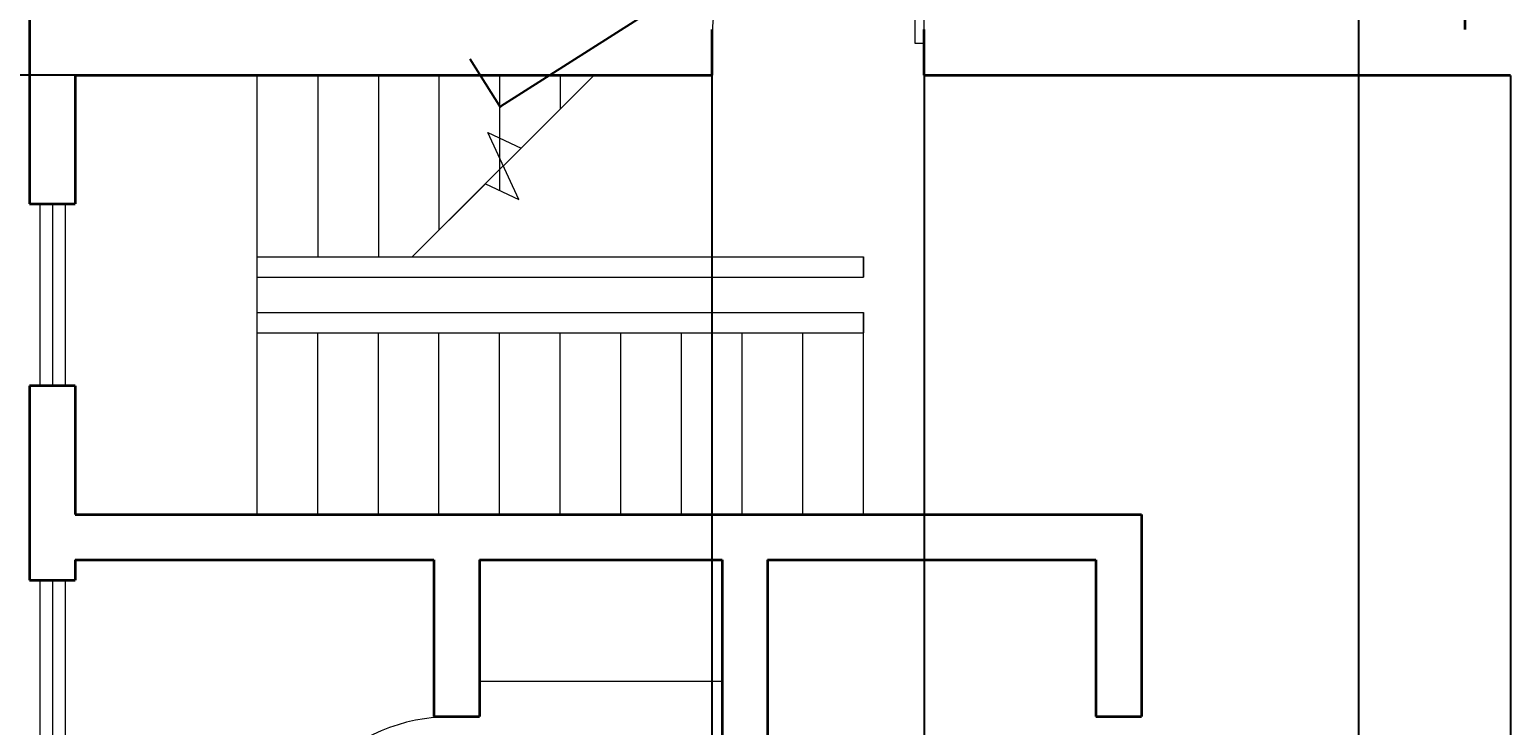
# Model space of a CAD drawing. Units: inches. Extents: x -4843 to -3402, y -164 to 3629.
# Tile 8 of 22: x -4596 to -4303, y 691 to 828. Entities that reach past the tile are written whole.
import ezdxf

# ---------------------------------------------------------------- set-up
doc = ezdxf.new("R2010")
doc.units = ezdxf.units.IN
for name, color, linetype, lineweight in [('A-ANNO-DIMS', 2, 'Continuous', 18), ('A-FLOR-CASE', 7, 'Continuous', 18), ('A-FLOR-STRS', 7, 'Continuous', 18), ('doors', 2, 'Continuous', 18), ('walls', 7, 'Continuous', 35), ('windows', 1, 'Continuous', 18)]:
    doc.layers.add(name, color=color, linetype=linetype, lineweight=lineweight)
doc.styles.get("Standard").update_dxf_attribs({"font": 'arial.ttf'})
doc.dimstyles.get("Standard").update_dxf_attribs({"dimtxt": 0.18, "dimasz": 0.18, "dimexe": 0.18, "dimexo": 0.0625, "dimgap": 0.09, "dimtad": 0, "dimtih": 1, "dimtoh": 1, "dimdec": 4, "dimzin": 0, "dimdsep": 46, "dimtxsty": 'Standard', "dimcen": 0.09, "dimadec": 0, "dimazin": 0, "dimtfac": 1, "dimtdec": 4, "dimtofl": 0, "dimtmove": 0, "dimatfit": 3, "dimfxl": 1, "dimtolj": 1, "dimtzin": 0, "dimarcsym": 0})

# ---------------------------------------------------------------- blocks, each defined once
blk = doc.blocks.new('windw 3')
at = {"layer": 'windows'}
for p, q in [((0, 7), (36, 7)), ((0, 4.5), (36, 4.5)), ((0, 2), (36, 2))]:
    blk.add_line(p, q, dxfattribs=at)
for points in [[(0, 0), (0, 9)], [(36, 9), (36, 0)]]:
    blk.add_lwpolyline(points, dxfattribs=at)
blk = doc.blocks.new('*U7')
for p, q in [((0, 0), (0, -6)), ((40, 0), (40, -6))]:
    blk.add_line(p, q)
blk.add_lwpolyline([(0, 0), (0, 40), (1.75, 40), (1.75, 0)], close=True)
blk.add_arc((0, 0), 40, 0, 90)
blk = doc.blocks.new('*U8')
for p, q in [((0, 0), (0, -6)), ((-40, 0), (-40, -6))]:
    blk.add_line(p, q)
blk.add_lwpolyline([(0, 0), (0, 40), (-1.75, 40), (-1.75, 0)], close=True)
blk.add_arc((0, 0), 40, 90, 180)
blk = doc.blocks.new('*D50')
at = {"layer": 'A-ANNO-DIMS', "color": 0, "lineweight": -2, "transparency": 16777216}
for p, q in [((-4445.31, 862.82), (-4439.2, 853.21)), ((-4439.45, 853.27), (-4470.7, 833.42)), ((-4502.52, 813.2), (-4471.27, 833.05)), ((-4508.68, 822.55), (-4502.58, 812.95))]:
    blk.add_line(p, q, dxfattribs=at)
at = {"layer": 'A-ANNO-DIMS', "color": 0, "transparency": 16777216}
for points in [[(-4439.47, 853.29), (-4439.43, 853.24), (-4439.3, 853.37)], [(-4502.54, 813.22), (-4502.51, 813.17), (-4502.67, 813.1)]]:
    blk.add_solid(points, dxfattribs=at)
at = {"layer": 'Defpoints', "color": 0, "transparency": 16777216}
for p in [(-4445.34, 862.87), (-4508.71, 822.61), (-4502.67, 813.1)]:
    blk.add_point(p, dxfattribs=at)
at = {"layer": 'A-ANNO-DIMS', "color": 0, "transparency": 16777216, "insert": (-4470.99, 833.23), "char_height": 0.18, "attachment_point": 5}
blk.add_mtext('\\A1;CHAIR SET 75', dxfattribs=at)
blk = doc.blocks.new('*D74')
at = {"layer": 'A-ANNO-DIMS', "color": 0, "lineweight": -2, "transparency": 16777216}
for p, q in [((-4595.85, 837.35), (-4842.55, 837.35)), ((-4842.37, 837.17), (-4842.37, 828.54)), ((-4842.37, 819.53), (-4842.37, 828.17)), ((-4586.85, 819.35), (-4842.55, 819.35))]:
    blk.add_line(p, q, dxfattribs=at)
at = {"layer": 'A-ANNO-DIMS', "color": 0, "transparency": 16777216}
for points in [[(-4842.4, 837.17), (-4842.34, 837.17), (-4842.37, 837.35)], [(-4842.4, 819.53), (-4842.34, 819.53), (-4842.37, 819.35)]]:
    blk.add_solid(points, dxfattribs=at)
at = {"layer": 'Defpoints', "color": 0, "transparency": 16777216}
for p in [(-4595.78, 837.35), (-4842.37, 819.35), (-4586.78, 819.35)]:
    blk.add_point(p, dxfattribs=at)
at = {"layer": 'A-ANNO-DIMS', "color": 0, "transparency": 16777216, "insert": (-4842.37, 828.35), "char_height": 0.18, "attachment_point": 5}
blk.add_mtext('\\A1;18', dxfattribs=at)
blk = doc.blocks.new('*D75')
at = {"layer": 'A-ANNO-DIMS', "color": 0, "lineweight": -2, "transparency": 16777216}
for p, q in [((-4460.78, 819.29), (-4460.78, 10.92)), ((-4418.78, 819.29), (-4418.78, 10.92)), ((-4460.6, 11.1), (-4440, 11.1)), ((-4418.96, 11.1), (-4439.56, 11.1))]:
    blk.add_line(p, q, dxfattribs=at)
at = {"layer": 'A-ANNO-DIMS', "color": 0, "transparency": 16777216}
for points in [[(-4460.6, 11.13), (-4460.6, 11.07), (-4460.78, 11.1)], [(-4418.96, 11.13), (-4418.96, 11.07), (-4418.78, 11.1)]]:
    blk.add_solid(points, dxfattribs=at)
at = {"layer": 'Defpoints', "color": 0, "transparency": 16777216}
for p in [(-4460.78, 819.35), (-4418.78, 819.35), (-4418.78, 11.1)]:
    blk.add_point(p, dxfattribs=at)
at = {"layer": 'A-ANNO-DIMS', "color": 0, "transparency": 16777216, "insert": (-4439.78, 11.1), "char_height": 0.18, "attachment_point": 5}
blk.add_mtext('\\A1;42', dxfattribs=at)
blk = doc.blocks.new('*D76')
at = {"layer": 'A-ANNO-DIMS', "color": 0, "lineweight": -2, "transparency": 16777216}
for p, q in [((-4418.78, 819.29), (-4418.78, 10.92)), ((-4302.78, 819.29), (-4302.78, 10.92)), ((-4418.6, 11.1), (-4361.06, 11.1)), ((-4302.96, 11.1), (-4360.5, 11.1))]:
    blk.add_line(p, q, dxfattribs=at)
at = {"layer": 'A-ANNO-DIMS', "color": 0, "transparency": 16777216}
for points in [[(-4418.6, 11.13), (-4418.6, 11.07), (-4418.78, 11.1)], [(-4302.96, 11.13), (-4302.96, 11.07), (-4302.78, 11.1)]]:
    blk.add_solid(points, dxfattribs=at)
at = {"layer": 'Defpoints', "color": 0, "transparency": 16777216}
for p in [(-4418.78, 819.35), (-4302.78, 819.35), (-4302.78, 11.1)]:
    blk.add_point(p, dxfattribs=at)
at = {"layer": 'A-ANNO-DIMS', "color": 0, "transparency": 16777216, "insert": (-4360.78, 11.1), "char_height": 0.18, "attachment_point": 5}
blk.add_mtext('\\A1;116', dxfattribs=at)
blk = doc.blocks.new('*D81')
at = {"layer": 'A-ANNO-DIMS', "color": 0, "lineweight": -2, "transparency": 16777216}
for p, q in [((-4332.78, 86.42), (-4332.78, 1392.95)), ((-4332.6, 1392.77), (-4168.61, 1392.77)), ((-4003.86, 1392.77), (-4167.86, 1392.77)), ((-4003.68, 86.42), (-4003.68, 1392.95))]:
    blk.add_line(p, q, dxfattribs=at)
at = {"layer": 'A-ANNO-DIMS', "color": 0, "transparency": 16777216}
for points in [[(-4332.6, 1392.8), (-4332.6, 1392.74), (-4332.78, 1392.77)], [(-4003.86, 1392.8), (-4003.86, 1392.74), (-4003.68, 1392.77)]]:
    blk.add_solid(points, dxfattribs=at)
at = {"layer": 'Defpoints', "color": 0, "transparency": 16777216}
for p in [(-4003.68, 1392.77), (-4332.78, 86.35), (-4003.68, 86.35)]:
    blk.add_point(p, dxfattribs=at)
at = {"layer": 'A-ANNO-DIMS', "color": 0, "transparency": 16777216, "insert": (-4168.23, 1392.77), "char_height": 0.18, "attachment_point": 5}
blk.add_mtext('\\A1;329.1', dxfattribs=at)

msp = doc.modelspace()

# ---------------------------------------------------------------- linework, layer by layer
at = {"layer": 'A-FLOR-CASE'}
msp.add_line((-4506.78, 699.35), (-4458.78, 699.35), dxfattribs=at)
at = {"layer": 'A-FLOR-STRS'}
for p, q in [((-4550.78, 732.35), (-4550.78, 819.35)), ((-4538.78, 819.35), (-4538.78, 783.35)), ((-4526.78, 819.35), (-4526.78, 783.35)), ((-4520.06, 783.35), (-4484.06, 819.35)), ((-4514.78, 819.35), (-4514.78, 788.63)), ((-4514.78, 819.35), (-4514.78, 788.63)), ((-4502.78, 819.35), (-4502.78, 796.51)), ((-4490.78, 819.35), (-4490.78, 812.63)), ((-4550.78, 783.35), (-4430.78, 783.35)), ((-4430.78, 783.35), (-4430.78, 779.35)), ((-4430.78, 779.35), (-4430.78, 783.35)), ((-4550.78, 779.35), (-4430.78, 779.35)), ((-4550.78, 772.35), (-4430.78, 772.35)), ((-4430.78, 732.35), (-4430.78, 772.35)), ((-4430.78, 772.35), (-4430.78, 768.35)), ((-4550.78, 768.35), (-4430.78, 768.35)), ((-4538.78, 732.35), (-4538.78, 768.35)), ((-4526.78, 732.35), (-4526.78, 768.35)), ((-4514.78, 732.35), (-4514.78, 768.35)), ((-4514.78, 732.35), (-4514.78, 768.35)), ((-4502.78, 732.35), (-4502.78, 768.35)), ((-4490.78, 732.35), (-4490.78, 768.35)), ((-4478.78, 732.35), (-4478.78, 768.35)), ((-4466.78, 732.35), (-4466.78, 768.35)), ((-4454.78, 732.35), (-4454.78, 768.35)), ((-4442.78, 732.35), (-4442.78, 768.35))]:
    msp.add_line(p, q, dxfattribs=at)
msp.add_lwpolyline([(-4520.06, 783.35), (-4505.59, 797.82), (-4498.97, 794.73), (-4505.14, 807.98), (-4498.52, 804.89), (-4484.06, 819.35)], dxfattribs=at)
at = {"layer": 'walls'}
for p, q in [((-4311.78, 894.35), (-4311.78, 828.35)), ((-4595.78, 837.35), (-4595.78, 793.85)), ((-4586.78, 819.35), (-4460.78, 819.35)), ((-4586.78, 819.35), (-4586.78, 793.85)), ((-4418.78, 819.35), (-4302.78, 819.35)), ((-4595.78, 757.85), (-4595.78, 739.35)), ((-4586.78, 757.85), (-4586.78, 732.35)), ((-4595.78, 739.35), (-4595.78, 719.35)), ((-4586.78, 732.35), (-4375.78, 732.35)), ((-4375.78, 732.35), (-4375.78, 692.35)), ((-4586.78, 723.35), (-4515.78, 723.35)), ((-4586.78, 723.35), (-4586.78, 719.35)), ((-4515.78, 723.35), (-4515.78, 692.35)), ((-4506.78, 723.35), (-4506.78, 692.35)), ((-4506.78, 723.35), (-4458.78, 723.35)), ((-4458.78, 723.35), (-4458.78, 643.35)), ((-4449.78, 723.35), (-4449.78, 652.35)), ((-4449.78, 723.35), (-4384.78, 723.35)), ((-4384.78, 723.35), (-4384.78, 692.35))]:
    msp.add_line(p, q, dxfattribs=at)
for points in [[(-4460.78, 828.35), (-4460.78, 819.35)], [(-4418.78, 819.35), (-4418.78, 828.35)], [(-4595.78, 793.85), (-4586.78, 793.85)], [(-4586.78, 757.85), (-4595.78, 757.85)], [(-4595.78, 719.35), (-4586.78, 719.35)], [(-4515.78, 692.35), (-4506.78, 692.35)], [(-4384.78, 692.35), (-4375.78, 692.35)]]:
    msp.add_lwpolyline(points, dxfattribs=at)

# ---------------------------------------------------------------- block references
at = {"layer": 'doors', "xscale": 1.05, "yscale": 1.05, "zscale": 1.05}
msp.add_blockref('*U8', (-4418.78, 825.65), dxfattribs=at)
at = {"layer": 'doors', "xscale": 0.9, "yscale": 0.9, "zscale": 0.9, "rotation": 90}
msp.add_blockref('*U7', (-4512.18, 656.35), dxfattribs=at)
at = {"layer": 'windows', "rotation": 270}
for p in [(-4595.78, 793.85), (-4595.78, 719.35)]:
    msp.add_blockref('windw 3', p, dxfattribs=at)

# ---------------------------------------------------------------- dimensions: what is measured, and where the dimension line sits
at = {"layer": 'A-ANNO-DIMS'}
for base, p1, p2, override, picture, middle in [((-4003.68, 1392.77), (-4332.78, 86.35), (-4003.68, 86.35), {"dimdec": 1, "dimlfac": 1, "dimrnd": 0, "dimzin": 0, "dimdsep": 46, "dimlunit": 2}, '*D81', (-4168.23, 1392.77)), ((-4418.78, 11.1), (-4460.78, 819.35), (-4418.78, 819.35), {"dimdec": 0, "dimlfac": 1, "dimrnd": 0, "dimzin": 0, "dimdsep": 46, "dimlunit": 2}, '*D75', (-4439.78, 11.1)), ((-4302.78, 11.1), (-4418.78, 819.35), (-4302.78, 819.35), {"dimdec": 0, "dimlfac": 1, "dimrnd": 0, "dimzin": 0, "dimdsep": 46, "dimlunit": 2}, '*D76', (-4360.78, 11.1))]:
    dim = msp.add_linear_dim(base=base, p1=p1, p2=p2, dimstyle='Standard', override=override, dxfattribs=at)
    dim.commit()
    dim.dimension.update_dxf_attribs({"geometry": picture, "text_midpoint": middle})
dim = msp.add_linear_dim(base=(-4502.67, 813.1), p1=(-4445.34, 862.87), p2=(-4508.71, 822.61), angle=212.4298, text='CHAIR SET <>', dimstyle='Standard', override={"dimdec": 0, "dimlfac": 1, "dimrnd": 0, "dimzin": 0, "dimdsep": 46, "dimlunit": 2}, dxfattribs=at)
dim.commit()
dim.dimension.update_dxf_attribs({"geometry": '*D50', "text_midpoint": (-4470.99, 833.23)})
dim = msp.add_linear_dim(base=(-4842.37, 819.35), p1=(-4595.78, 837.35), p2=(-4586.78, 819.35), angle=90, dimstyle='Standard', override={"dimdec": 0, "dimlfac": 1, "dimrnd": 0, "dimzin": 0, "dimdsep": 46, "dimlunit": 2}, dxfattribs=at)
dim.commit()
dim.dimension.update_dxf_attribs({"geometry": '*D74', "text_midpoint": (-4842.37, 828.35)})

doc.saveas('drawing.dxf')
